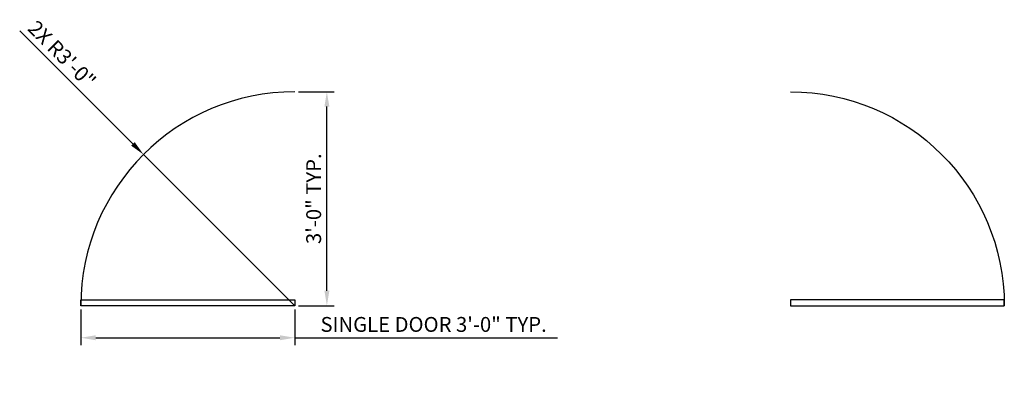
# Model space of a CAD drawing. Units: inches. Extents: x 877 to 2164, y 771 to 1603.
# Tile 6 of 6: x 1999 to 2164, y 1544 to 1603. Entities that reach past the tile are written whole.
import ezdxf

# ---------------------------------------------------------------- set-up
doc = ezdxf.new("R2010")
doc.units = ezdxf.units.IN
doc.layers.add('A-ANNO-DIMS', color=2, linetype='Continuous', lineweight=18)
doc.layers.add('A-DOOR', color=5, linetype='Continuous', lineweight=25)
doc.styles.get("Standard").update_dxf_attribs({"font": 'arial.ttf'})
doc.dimstyles.new('ISO-25', dxfattribs={"dimtxt": 2.5, "dimasz": 2.5, "dimexe": 1.25, "dimexo": 0.625, "dimtad": 1, "dimdec": 0, "dimlunit": 4, "dimtxsty": 'Standard', "dimcen": 2.5, "dimadec": 0, "dimazin": 0, "dimtfac": 1, "dimtdec": 0, "dimtmove": 0, "dimatfit": 3, "dimfxl": 1, "dimarcsym": 0})

# ---------------------------------------------------------------- blocks, each defined once
blk = doc.blocks.new('DOOR-SINGLE-36IN')
blk.add_lwpolyline([(0, 0), (0, 1), (36, 1), (36, 0)], close=True)
blk.add_arc((36, 0), 36, 90, 180)
blk = doc.blocks.new('*D6')
at = {"layer": 'A-ANNO-DIMS', "color": 0, "lineweight": -2, "transparency": 16777216}
for p, q in [((2008.9, 1554.37), (2008.9, 1548.34)), ((2044.9, 1554.37), (2044.9, 1548.34)), ((2011.4, 1549.59), (2042.4, 1549.59)), ((2044.9, 1549.59), (2089.11, 1549.59))]:
    blk.add_line(p, q, dxfattribs=at)
at = {"layer": 'A-ANNO-DIMS', "color": 0, "transparency": 16777216}
for points in [[(2011.4, 1550.01), (2011.4, 1549.17), (2008.9, 1549.59)], [(2042.4, 1550.01), (2042.4, 1549.17), (2044.9, 1549.59)]]:
    blk.add_solid(points, dxfattribs=at)
at = {"layer": 'Defpoints', "color": 0, "transparency": 16777216}
for p in [(2008.9, 1554.99), (2044.9, 1554.99), (2044.9, 1549.59)]:
    blk.add_point(p, dxfattribs=at)
at = {"layer": 'A-ANNO-DIMS', "color": 0, "transparency": 16777216, "insert": (2068.26, 1551.51), "char_height": 2.5, "attachment_point": 5}
blk.add_mtext('SINGLE DOOR 3\'-0" TYP.', dxfattribs=at)
blk = doc.blocks.new('*D7')
at = {"layer": 'A-ANNO-DIMS', "color": 0, "lineweight": -2, "transparency": 16777216}
for p, q in [((2045.53, 1590.99), (2051.55, 1590.99)), ((2050.3, 1557.49), (2050.3, 1588.49)), ((2045.53, 1554.99), (2051.55, 1554.99))]:
    blk.add_line(p, q, dxfattribs=at)
at = {"layer": 'A-ANNO-DIMS', "color": 0, "transparency": 16777216}
for points in [[(2049.89, 1588.49), (2050.72, 1588.49), (2050.3, 1590.99)], [(2049.89, 1557.49), (2050.72, 1557.49), (2050.3, 1554.99)]]:
    blk.add_solid(points, dxfattribs=at)
at = {"layer": 'Defpoints', "color": 0, "transparency": 16777216}
for p in [(2044.9, 1590.99), (2050.3, 1590.99), (2044.9, 1554.99)]:
    blk.add_point(p, dxfattribs=at)
at = {"layer": 'A-ANNO-DIMS', "color": 0, "transparency": 16777216, "insert": (2048.4, 1572.99), "char_height": 2.5, "attachment_point": 5, "rotation": 90}
blk.add_mtext('3\'-0" TYP.', dxfattribs=at)
blk = doc.blocks.new('*D47')
at = {"layer": 'A-ANNO-DIMS', "color": 0, "lineweight": -2, "transparency": 16777216}
for p, q in [((1998.61, 1601.26), (2017.67, 1582.21)), ((2044.9, 1554.99), (2019.44, 1580.44))]:
    blk.add_line(p, q, dxfattribs=at)
at = {"layer": 'A-ANNO-DIMS', "color": 0, "transparency": 16777216}
blk.add_solid([(2017.97, 1582.5), (2017.38, 1581.91), (2019.44, 1580.44)], dxfattribs=at)
at = {"layer": 'Defpoints', "color": 0, "transparency": 16777216}
for p in [(2019.44, 1580.44), (2044.9, 1554.99)]:
    blk.add_point(p, dxfattribs=at)
at = {"layer": 'A-ANNO-DIMS', "color": 0, "transparency": 16777216, "insert": (2005.51, 1597.05), "char_height": 2.5, "attachment_point": 5, "rotation": 315.0158}
blk.add_mtext('2X R3\'-0"', dxfattribs=at)

msp = doc.modelspace()

# ---------------------------------------------------------------- block references
at = {"layer": 'A-DOOR'}
msp.add_blockref('DOOR-SINGLE-36IN', (2008.9, 1554.99), dxfattribs=at)
at = {"layer": 'A-DOOR', "extrusion": (0, 0, -1), "zscale": -1}
msp.add_blockref('DOOR-SINGLE-36IN', (-2164.3, 1554.99), dxfattribs=at)

# ---------------------------------------------------------------- dimensions: what is measured, and where the dimension line sits
at = {"layer": 'A-ANNO-DIMS'}
dim = msp.add_radius_dim(center=(2044.9, 1554.99), mpoint=(2019.44, 1580.44), text='2X <>', dimstyle='ISO-25', override={"dimdec": 1, "dimlfac": 1, "dimrnd": 0, "dimzin": 1, "dimdsep": 46, "dimlunit": 4, "dimfrac": 2}, dxfattribs=at)
dim.commit()
dim.dimension.update_dxf_attribs({"geometry": '*D47', "text_midpoint": (2004.16, 1595.71), "dimtype": 164})
dim = msp.add_linear_dim(base=(2050.3, 1590.99), p1=(2044.9, 1554.99), p2=(2044.9, 1590.99), angle=90, text='<> TYP.', dimstyle='ISO-25', override={"dimdec": 1, "dimlfac": 1, "dimrnd": 0, "dimzin": 1, "dimdsep": 46, "dimlunit": 4, "dimfrac": 2}, dxfattribs=at)
dim.commit()
dim.dimension.update_dxf_attribs({"geometry": '*D7', "text_midpoint": (2048.4, 1572.99)})
dim = msp.add_linear_dim(base=(2044.9, 1549.59), p1=(2008.9, 1554.99), p2=(2044.9, 1554.99), text='SINGLE DOOR <> TYP.', dimstyle='ISO-25', override={"dimdec": 1, "dimlfac": 1, "dimrnd": 0, "dimzin": 1, "dimdsep": 46, "dimlunit": 4, "dimfrac": 2}, dxfattribs=at)
dim.commit()
dim.dimension.update_dxf_attribs({"geometry": '*D6', "text_midpoint": (2068.26, 1551.51)})

doc.saveas('drawing.dxf')
